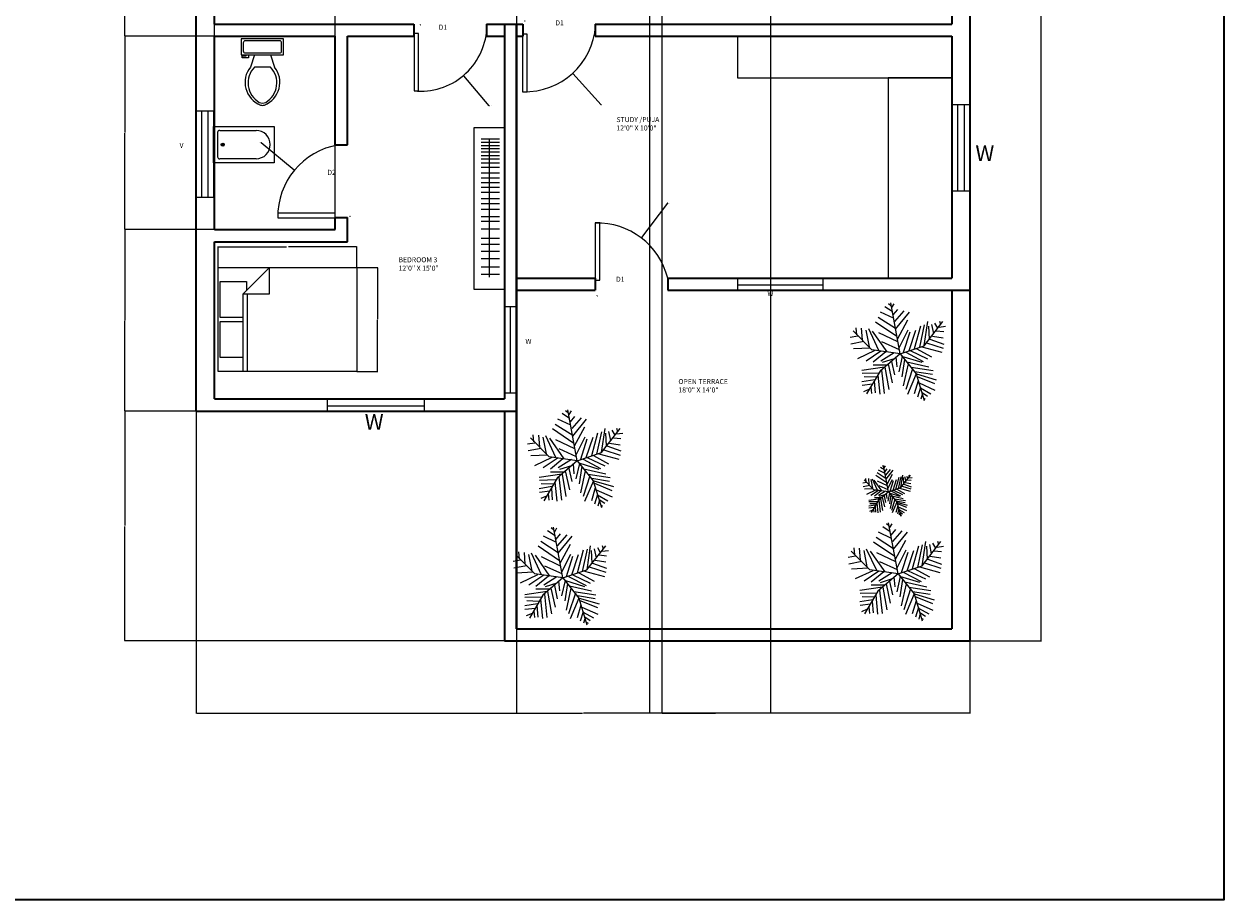
# Model space of a CAD drawing. Units: inches. Extents: x 65 to 1274, y 42 to 1041.
# Tile 4 of 6: x 678 to 1274, y 42 to 476. Entities that reach past the tile are written whole.
import ezdxf

# ---------------------------------------------------------------- set-up
doc = ezdxf.new("R2010")
doc.units = ezdxf.units.IN
for name, color, linetype, lineweight in [('A-ANNO-DIMS', 2, 'Continuous', 18), ('A-AREA-IDEN', 7, 'Continuous', 18), ('A-DOOR', 3, 'Continuous', 18), ('A-FLOR-CASE', 8, 'Continuous', 18), ('A-FLOR-FIXT', 9, 'Continuous', 18), ('A-FURN', 8, 'Continuous', 18), ('A-GLAZ', 4, 'Continuous', 18), ('A-WALL', 7, 'Continuous', 35), ('L-PLNT', 94, 'Continuous', 13), ('Text', 7, 'Continuous', 18), ('Title Block', 7, 'Continuous', 35)]:
    doc.layers.add(name, color=color, linetype=linetype, lineweight=lineweight)
doc.styles.get("Standard").update_dxf_attribs({"font": 'arial.ttf'})
doc.dimstyles.get("Standard").update_dxf_attribs({"dimtxt": 0.18, "dimasz": 0.18, "dimexe": 0.18, "dimexo": 0.0625, "dimgap": 0.09, "dimtad": 0, "dimtih": 1, "dimtoh": 1, "dimdec": 4, "dimzin": 0, "dimdsep": 46, "dimtxsty": 'Standard', "dimcen": 0.09, "dimadec": 0, "dimazin": 0, "dimtfac": 1, "dimtdec": 4, "dimtofl": 0, "dimtmove": 0, "dimatfit": 3, "dimfxl": 1, "dimtolj": 1, "dimtzin": 0, "dimarcsym": 0})

# ---------------------------------------------------------------- blocks, each defined once
blk = doc.blocks.new('Toilet - top')
for p, q in [((9.5, -6), (9.5, -2)), ((-10, -8.5), (-8, -8.5)), ((-10, -9.5), (-10, -8.5)), ((-7, -9.5), (-10, -9.5)), ((-8, -8.5), (-8, -8)), ((-7, -8), (-7, -9.5)), ((-4, -8), (-6, -14)), ((4, -8), (6, -14)), ((4, -14), (-4, -14))]:
    blk.add_line(p, q)
blk.add_lwpolyline([(10.5, -8), (10.5, 0), (-10.5, 0), (-10.5, -8)], close=True)
for points in [[(-9.5, -2), (-9.5, -6)], [(8.5, -1), (-8.5, -1)], [(-8.5, -7), (8.5, -7)]]:
    blk.add_lwpolyline(points)
for centre, radius, start, end in [((-8.62, -1.88), 0.884, 81.8699, 188.1301), ((8.62, -1.88), 0.884, 351.8699, 98.1301), ((-8.62, -6.12), 0.884, 171.8699, 278.1301), ((8.62, -6.12), 0.884, 261.8699, 8.1301), ((3.52, -21.58), 12.17, 141.46911, 247.97143), ((4.2, -21.82), 11.33, 136.36773, 238.94682), ((-3.52, -21.58), 12.17, 292.02843, 38.53071), ((-4.2, -21.82), 11.33, 301.05301, 43.63209), ((0, -27.88), 4, 245.73182, 294.26817), ((0, -29), 4, 254.86053, 285.13947)]:
    blk.add_arc(centre, radius, start, end)
blk = doc.blocks.new('Bath Tub - 26 x 60 in.')
for p, q in [((8, -18), (10, -18)), ((9, -17), (9, -19))]:
    blk.add_line(p, q)
blk.add_lwpolyline([(0, -36), (0, 0), (60, 0), (60, -36)], close=True)
for points in [[(4, -30), (4, -6)], [(6, -4), (42, -4)], [(42, -32), (6, -32)]]:
    blk.add_lwpolyline(points)
for radius in [1.5, 1]:
    blk.add_circle((9, -18), radius)
for centre, radius, start, end in [((5.75, -5.75), 1.77, 81.8699, 188.1301), ((42, -18), 14, 270, 90), ((5.75, -30.25), 1.77, 171.8699, 278.1301)]:
    blk.add_arc(centre, radius, start, end)
blk = doc.blocks.new('Bed - Queen')
for p, q in [((0, -80.00003), (0, 0)), ((0, 0), (59.99999, 0)), ((59.99999, 0), (59.99999, -80.00003)), ((7.99999, -1.2), (28.79998, -1.2)), ((7.99999, -14.4), (7.99999, -1.2)), ((28.79998, -1.2), (28.79998, -14.4)), ((31.19999, -1.2), (51.99999, -1.2)), ((31.19999, -14.4), (31.19999, -1.2)), ((51.99999, -1.2), (51.99999, -16.4)), ((0, -14.4), (44.8, -14.4)), ((44.8, -16.8), (0, -16.8)), ((59.99999, -29.6), (44.8, -14.4)), ((44.8, -14.4), (44.8, -29.6)), ((51.99999, -16.4), (46.79936, -16.4)), ((44.8, -29.6), (59.99999, -29.6)), ((59.99999, -80.00003), (0, -80.00003))]:
    blk.add_line(p, q)
blk = doc.blocks.new('*U4')
for p, q in [((-10.186, 53.64), (-13.084, 55.962)), ((0, 0), (-10.5, 57)), ((-9.099, 51.782), (-6.563, 55.962)), ((-5.114, 28.097), (-24.676, 40.636)), ((-7.288, 39.707), (-21.778, 46.673)), ((-8.737, 47.138), (-17.069, 52.711)), ((-7.65, 43.423), (-2.578, 49.46)), ((-5.839, 35.992), (4.667, 48.067)), ((-5.114, 27.632), (10.463, 46.673)), ((-48.585, 21.131), (-49.309, 29.026)), ((-43.513, 28.561), (-42.427, 15.558)), ((-35.544, 28.097), (-24.314, 3.947)), ((-3.665, 19.273), (-27.574, 35.527)), ((-2.941, 16.486), (8.652, 37.85)), ((16.259, 5.805), (23.142, 31.348)), ((22.055, 7.198), (27.489, 32.277)), ((27, 9), (48, 36)), ((27.127, 9.056), (31.112, 35.992)), ((31.836, 30.883), (32.561, 16.486)), ((35.096, 32.741), (37.27, 22.524)), ((38.719, 34.134), (41.979, 28.561)), ((43.791, 29.954), (51.036, 30.883)), ((44.153, 36.456), (45.239, 32.741)), ((-47.498, 19.737), (-55.83, 18.344)), ((-40.615, 13.7), (-55.105, 10.913)), ((-31.5, 4.5), (-52.5, 25.5)), ((-38.442, 26.239), (-34.819, 7.663)), ((-14.533, 2.09), (-30.834, 25.31)), ((-24.314, 23.917), (-2.941, 13.7)), ((-20.691, 13.7), (-1.129, 4.876)), ((-1.129, 6.734), (9.014, 26.704)), ((3.942, 1.625), (11.187, 24.381)), ((10.101, 3.483), (17.708, 26.239)), ((33.285, 16.486), (48.862, 10.913)), ((36.183, 19.737), (48.137, 17.88)), ((40.53, 25.775), (48.862, 24.846)), ((-33.37, 6.269), (-52.207, 5.34)), ((-28.299, 3.483), (-47.86, -5.805)), ((-21.416, 3.018), (-38.079, -8.128)), ((0, 0), (-31.5, 4.5)), ((-15.982, 2.09), (-30.11, -9.521)), ((0, 0), (-22.5, -19.5)), ((-6.563, 1.161), (-21.416, -8.128)), ((0, 0), (27, 9)), ((0, 0), (18, -22.5)), ((6.478, 1.625), (26.04, -8.592)), ((11.187, 3.483), (30.749, -5.805)), ((18.07, 5.805), (35.096, -3.483)), ((24.229, 7.663), (46.688, 1.625)), ((29.662, 12.307), (48.137, 6.269)), ((-15.257, -12.772), (-30.11, -12.772)), ((-6.563, -5.805), (-19.967, -9.985)), ((-13.446, -11.378), (-8.737, -32.741)), ((-9.461, -8.592), (-6.201, -23.453)), ((-4.752, -3.483), (-3.665, -14.629)), ((2.493, -3.019), (-1.491, -20.202)), ((1.769, -2.555), (24.229, -9.521)), ((5.029, -6.27), (2.131, -25.775)), ((9.014, -11.378), (3.58, -35.992)), ((7.565, -9.056), (32.198, -14.629)), ((-17.431, -15.094), (-42.789, -18.809)), ((-24.314, -21.596), (-42.427, -22.06)), ((-26.849, -26.24), (-40.253, -25.775)), ((-22.5, -19.5), (-37.5, -45)), ((-25.038, -23.918), (-22.865, -45.281)), ((-20.691, -18.345), (-17.793, -44.352)), ((-17.069, -15.094), (-12.721, -40.172)), ((14.085, -16.951), (6.478, -40.172)), ((18.07, -22.524), (8.289, -45.745)), ((12.274, -15.094), (36.907, -18.809)), ((16.259, -19.738), (36.183, -22.989)), ((18, -22.5), (27, -52.5)), ((18.433, -22.524), (40.53, -29.026)), ((19.157, -25.311), (38.719, -33.206)), ((-28.299, -29.026), (-42.789, -31.348)), ((-30.834, -34.135), (-42.427, -35.528)), ((-34.457, -39.708), (-40.978, -42.494)), ((-32.646, -36.921), (-31.921, -44.352)), ((-29.023, -30.884), (-27.936, -43.887)), ((20.244, -30.419), (15.897, -44.816)), ((22.78, -37.85), (19.519, -48.532)), ((21.331, -32.741), (39.081, -40.636)), ((22.78, -38.314), (34.372, -44.816)), ((24.591, -45.745), (23.142, -50.854)), ((24.591, -43.423), (30.749, -47.603)), ((26.764, -49.925), (28.213, -50.854))]:
    blk.add_line(p, q)
blk = doc.blocks.new('WIN-43-DEEP-FRAME')
for p, q in [((9, 42.65), (0, 42.65)), ((0, 42.65), (0, 0)), ((3, 0), (3, 42.65)), ((6, 42.65), (6, 0)), ((9, 0), (9, 42.65)), ((0, 0), (9, 0))]:
    blk.add_line(p, q)
blk = doc.blocks.new('*D30')
at = {"layer": 'A-ANNO-DIMS', "color": 0, "lineweight": -2, "transparency": 16777216}
for p, q in [((774.7, 355.42), (774.7, 365.85)), ((774.88, 365.67), (808.56, 365.67)), ((843.26, 365.67), (809.58, 365.67)), ((843.44, 355.42), (843.44, 365.85))]:
    blk.add_line(p, q, dxfattribs=at)
at = {"layer": 'A-ANNO-DIMS', "color": 0, "transparency": 16777216}
for points in [[(774.88, 365.7), (774.88, 365.64), (774.7, 365.67)], [(843.26, 365.7), (843.26, 365.64), (843.44, 365.67)]]:
    blk.add_solid(points, dxfattribs=at)
at = {"layer": 'Defpoints', "color": 0, "transparency": 16777216}
for p in [(774.7, 365.67), (774.7, 355.36), (843.44, 355.36)]:
    blk.add_point(p, dxfattribs=at)
at = {"layer": 'A-ANNO-DIMS', "color": 0, "transparency": 16777216, "insert": (809.07, 365.67), "char_height": 0.18, "attachment_point": 5}
blk.add_mtext('\\A1;BED 69', dxfattribs=at)
blk = doc.blocks.new('*D31')
at = {"layer": 'A-ANNO-DIMS', "color": 0, "lineweight": -2, "transparency": 16777216}
for p, q in [((843.5, 355.36), (853.93, 355.36)), ((853.75, 355.18), (853.75, 329.76)), ((853.75, 303.99), (853.75, 329.4)), ((843.5, 303.81), (853.93, 303.81))]:
    blk.add_line(p, q, dxfattribs=at)
at = {"layer": 'A-ANNO-DIMS', "color": 0, "transparency": 16777216}
for points in [[(853.72, 355.18), (853.78, 355.18), (853.75, 355.36)], [(853.72, 303.99), (853.78, 303.99), (853.75, 303.81)]]:
    blk.add_solid(points, dxfattribs=at)
at = {"layer": 'Defpoints', "color": 0, "transparency": 16777216}
for p in [(843.44, 355.36), (853.75, 355.36), (843.44, 303.81)]:
    blk.add_point(p, dxfattribs=at)
at = {"layer": 'A-ANNO-DIMS', "color": 0, "transparency": 16777216, "insert": (853.75, 329.58), "char_height": 0.18, "attachment_point": 5}
blk.add_mtext('\\A1;52', dxfattribs=at)
blk = doc.blocks.new('*D64')
at = {"layer": 'A-ANNO-DIMS', "color": 0, "lineweight": -2, "transparency": 16777216}
for p, q in [((763.83, 284.09), (763.83, 134.18)), ((1147.83, 170.09), (1147.83, 134.18)), ((764.01, 134.36), (955.54, 134.36)), ((1147.65, 134.36), (956.12, 134.36))]:
    blk.add_line(p, q, dxfattribs=at)
at = {"layer": 'A-ANNO-DIMS', "color": 0, "transparency": 16777216}
for points in [[(764.01, 134.39), (764.01, 134.33), (763.83, 134.36)], [(1147.65, 134.39), (1147.65, 134.33), (1147.83, 134.36)]]:
    blk.add_solid(points, dxfattribs=at)
at = {"layer": 'Defpoints', "color": 0, "transparency": 16777216}
for p in [(763.83, 284.15), (1147.83, 170.15), (1147.83, 134.36)]:
    blk.add_point(p, dxfattribs=at)
at = {"layer": 'A-ANNO-DIMS', "color": 0, "transparency": 16777216, "insert": (955.83, 134.36), "char_height": 0.18, "attachment_point": 5}
blk.add_mtext('\\A1;384', dxfattribs=at)
blk = doc.blocks.new('*D65')
at = {"layer": 'A-ANNO-DIMS', "color": 0, "lineweight": -2, "transparency": 16777216}
for p, q in [((1147.89, 827.15), (1183.32, 827.15)), ((1183.14, 826.97), (1183.14, 498.83)), ((1183.14, 170.33), (1183.14, 498.47)), ((1147.89, 170.15), (1183.32, 170.15))]:
    blk.add_line(p, q, dxfattribs=at)
at = {"layer": 'A-ANNO-DIMS', "color": 0, "transparency": 16777216}
for points in [[(1183.11, 826.97), (1183.17, 826.97), (1183.14, 827.15)], [(1183.11, 170.33), (1183.17, 170.33), (1183.14, 170.15)]]:
    blk.add_solid(points, dxfattribs=at)
at = {"layer": 'Defpoints', "color": 0, "transparency": 16777216}
for p in [(1147.83, 827.15), (1183.14, 827.15), (1147.83, 170.15)]:
    blk.add_point(p, dxfattribs=at)
at = {"layer": 'A-ANNO-DIMS', "color": 0, "transparency": 16777216, "insert": (1183.14, 498.65), "char_height": 0.18, "attachment_point": 5}
blk.add_mtext('\\A1;657', dxfattribs=at)
blk = doc.blocks.new('*D68')
at = {"layer": 'A-ANNO-DIMS', "color": 0, "lineweight": -2, "transparency": 16777216}
for p, q in [((922.83, 722.09), (922.83, 134.18)), ((988.83, 722.09), (988.83, 134.18)), ((923.01, 134.36), (955.61, 134.36)), ((988.65, 134.36), (956.05, 134.36))]:
    blk.add_line(p, q, dxfattribs=at)
at = {"layer": 'A-ANNO-DIMS', "color": 0, "transparency": 16777216}
for points in [[(923.01, 134.39), (923.01, 134.33), (922.83, 134.36)], [(988.65, 134.39), (988.65, 134.33), (988.83, 134.36)]]:
    blk.add_solid(points, dxfattribs=at)
at = {"layer": 'Defpoints', "color": 0, "transparency": 16777216}
for p in [(922.83, 722.15), (988.83, 722.15), (988.83, 134.36)]:
    blk.add_point(p, dxfattribs=at)
at = {"layer": 'A-ANNO-DIMS', "color": 0, "transparency": 16777216, "insert": (955.83, 134.36), "char_height": 0.18, "attachment_point": 5}
blk.add_mtext('\\A1;66', dxfattribs=at)
blk = doc.blocks.new('*D69')
at = {"layer": 'A-ANNO-DIMS', "color": 0, "lineweight": -2, "transparency": 16777216}
for p, q in [((994.83, 722.09), (994.83, 134.18)), ((1048.83, 722.09), (1048.83, 134.18)), ((995.01, 134.36), (1021.61, 134.36)), ((1048.65, 134.36), (1022.05, 134.36))]:
    blk.add_line(p, q, dxfattribs=at)
at = {"layer": 'A-ANNO-DIMS', "color": 0, "transparency": 16777216}
for points in [[(995.01, 134.39), (995.01, 134.33), (994.83, 134.36)], [(1048.65, 134.39), (1048.65, 134.33), (1048.83, 134.36)]]:
    blk.add_solid(points, dxfattribs=at)
at = {"layer": 'Defpoints', "color": 0, "transparency": 16777216}
for p in [(994.83, 722.15), (1048.83, 722.15), (1048.83, 134.36)]:
    blk.add_point(p, dxfattribs=at)
at = {"layer": 'A-ANNO-DIMS', "color": 0, "transparency": 16777216, "insert": (1021.83, 134.36), "char_height": 0.18, "attachment_point": 5}
blk.add_mtext('\\A1;54', dxfattribs=at)
blk = doc.blocks.new('*D70')
at = {"layer": 'A-ANNO-DIMS', "color": 0, "lineweight": -2, "transparency": 16777216}
for p, q in [((763.77, 284.15), (728.22, 284.15)), ((728.4, 283.97), (728.4, 227.33)), ((728.4, 170.33), (728.4, 226.97)), ((916.77, 170.15), (728.22, 170.15))]:
    blk.add_line(p, q, dxfattribs=at)
at = {"layer": 'A-ANNO-DIMS', "color": 0, "transparency": 16777216}
for points in [[(728.37, 283.97), (728.43, 283.97), (728.4, 284.15)], [(728.37, 170.33), (728.43, 170.33), (728.4, 170.15)]]:
    blk.add_solid(points, dxfattribs=at)
at = {"layer": 'Defpoints', "color": 0, "transparency": 16777216}
for p in [(728.4, 284.15), (763.83, 284.15), (916.83, 170.15)]:
    blk.add_point(p, dxfattribs=at)
at = {"layer": 'A-ANNO-DIMS', "color": 0, "transparency": 16777216, "insert": (728.4, 227.15), "char_height": 0.18, "attachment_point": 5}
blk.add_mtext('\\A1;114', dxfattribs=at)
blk = doc.blocks.new('*D71')
at = {"layer": 'A-ANNO-DIMS', "color": 0, "lineweight": -2, "transparency": 16777216}
for p, q in [((772.77, 374.15), (728.22, 374.15)), ((728.4, 373.97), (728.4, 329.33)), ((728.4, 284.33), (728.4, 328.97)), ((763.77, 284.15), (728.22, 284.15))]:
    blk.add_line(p, q, dxfattribs=at)
at = {"layer": 'A-ANNO-DIMS', "color": 0, "transparency": 16777216}
for points in [[(728.37, 373.97), (728.43, 373.97), (728.4, 374.15)], [(728.37, 284.33), (728.43, 284.33), (728.4, 284.15)]]:
    blk.add_solid(points, dxfattribs=at)
at = {"layer": 'Defpoints', "color": 0, "transparency": 16777216}
for p in [(728.4, 374.15), (772.83, 374.15), (763.83, 284.15)]:
    blk.add_point(p, dxfattribs=at)
at = {"layer": 'A-ANNO-DIMS', "color": 0, "transparency": 16777216, "insert": (728.4, 329.15), "char_height": 0.18, "attachment_point": 5}
blk.add_mtext('\\A1;90', dxfattribs=at)
blk = doc.blocks.new('*D72')
at = {"layer": 'A-ANNO-DIMS', "color": 0, "lineweight": -2, "transparency": 16777216}
for p, q in [((772.77, 470.15), (728.22, 470.15)), ((728.4, 469.97), (728.4, 422.33)), ((728.4, 374.33), (728.4, 421.97)), ((772.77, 374.15), (728.22, 374.15))]:
    blk.add_line(p, q, dxfattribs=at)
at = {"layer": 'A-ANNO-DIMS', "color": 0, "transparency": 16777216}
for points in [[(728.37, 469.97), (728.43, 469.97), (728.4, 470.15)], [(728.37, 374.33), (728.43, 374.33), (728.4, 374.15)]]:
    blk.add_solid(points, dxfattribs=at)
at = {"layer": 'Defpoints', "color": 0, "transparency": 16777216}
for p in [(728.4, 470.15), (772.83, 470.15), (772.83, 374.15)]:
    blk.add_point(p, dxfattribs=at)
at = {"layer": 'A-ANNO-DIMS', "color": 0, "transparency": 16777216, "insert": (728.4, 422.15), "char_height": 0.18, "attachment_point": 5}
blk.add_mtext('\\A1;96', dxfattribs=at)
blk = doc.blocks.new('*D73')
at = {"layer": 'A-ANNO-DIMS', "color": 0, "lineweight": -2, "transparency": 16777216}
for p, q in [((772.48, 549.58), (728.22, 549.58)), ((728.4, 549.4), (728.4, 510.05)), ((728.4, 470.33), (728.4, 509.68)), ((772.77, 470.15), (728.22, 470.15))]:
    blk.add_line(p, q, dxfattribs=at)
at = {"layer": 'A-ANNO-DIMS', "color": 0, "transparency": 16777216}
for points in [[(728.37, 549.4), (728.43, 549.4), (728.4, 549.58)], [(728.37, 470.33), (728.43, 470.33), (728.4, 470.15)]]:
    blk.add_solid(points, dxfattribs=at)
at = {"layer": 'Defpoints', "color": 0, "transparency": 16777216}
for p in [(728.4, 549.58), (772.55, 549.58), (772.83, 470.15)]:
    blk.add_point(p, dxfattribs=at)
at = {"layer": 'A-ANNO-DIMS', "color": 0, "transparency": 16777216, "insert": (728.4, 509.86), "char_height": 0.18, "attachment_point": 5}
blk.add_mtext('\\A1;79.43', dxfattribs=at)
blk = doc.blocks.new('*D77')
at = {"layer": 'A-ANNO-DIMS', "color": 0, "lineweight": -2, "transparency": 16777216}
for p, q in [((772.83, 374.21), (772.83, 890.96)), ((773.01, 890.78), (802.61, 890.78)), ((832.65, 890.78), (803.05, 890.78)), ((832.83, 374.21), (832.83, 890.96))]:
    blk.add_line(p, q, dxfattribs=at)
at = {"layer": 'A-ANNO-DIMS', "color": 0, "transparency": 16777216}
for points in [[(773.01, 890.81), (773.01, 890.75), (772.83, 890.78)], [(832.65, 890.81), (832.65, 890.75), (832.83, 890.78)]]:
    blk.add_solid(points, dxfattribs=at)
at = {"layer": 'Defpoints', "color": 0, "transparency": 16777216}
for p in [(832.83, 890.78), (772.83, 374.15), (832.83, 374.15)]:
    blk.add_point(p, dxfattribs=at)
at = {"layer": 'A-ANNO-DIMS', "color": 0, "transparency": 16777216, "insert": (802.83, 890.78), "char_height": 0.18, "attachment_point": 5}
blk.add_mtext('\\A1;60', dxfattribs=at)
blk = doc.blocks.new('*D84')
at = {"layer": 'A-ANNO-DIMS', "color": 0, "lineweight": -2, "transparency": 16777216}
for p, q in [((875.01, 475.78), (875.19, 475.78)), ((875.1, 475.69), (875.1, 475.87)), ((909.25, 435.54), (896.56, 450.49)), ((909.43, 435.54), (909.25, 435.54))]:
    blk.add_line(p, q, dxfattribs=at)
at = {"layer": 'A-ANNO-DIMS', "color": 0, "transparency": 16777216}
blk.add_solid([(896.59, 450.51), (896.54, 450.47), (896.45, 450.63)], dxfattribs=at)
at = {"layer": 'Defpoints', "color": 0, "transparency": 16777216}
for p in [(875.1, 475.78), (896.45, 450.63)]:
    blk.add_point(p, dxfattribs=at)
at = {"layer": 'A-ANNO-DIMS', "color": 0, "transparency": 16777216, "insert": (909.91, 435.54), "char_height": 0.18, "attachment_point": 5}
blk.add_mtext('\\A1;R32.99', dxfattribs=at)
blk = doc.blocks.new('*D85')
at = {"layer": 'A-ANNO-DIMS', "color": 0, "lineweight": -2, "transparency": 16777216}
for p, q in [((926.86, 477.66), (927.04, 477.66)), ((926.95, 477.57), (926.95, 477.75)), ((964.73, 436.07), (950.68, 451.53)), ((964.91, 436.07), (964.73, 436.07))]:
    blk.add_line(p, q, dxfattribs=at)
at = {"layer": 'A-ANNO-DIMS', "color": 0, "transparency": 16777216}
blk.add_solid([(950.7, 451.55), (950.66, 451.51), (950.56, 451.66)], dxfattribs=at)
at = {"layer": 'Defpoints', "color": 0, "transparency": 16777216}
for p in [(926.95, 477.66), (950.56, 451.66)]:
    blk.add_point(p, dxfattribs=at)
at = {"layer": 'A-ANNO-DIMS', "color": 0, "transparency": 16777216, "insert": (965.46, 436.07), "char_height": 0.18, "attachment_point": 5}
blk.add_mtext('\\A1;R35.115', dxfattribs=at)
blk = doc.blocks.new('*D86')
at = {"layer": 'A-ANNO-DIMS', "color": 0, "lineweight": -2, "transparency": 16777216}
for p, q in [((795.81, 417.41), (795.99, 417.41)), ((795.99, 417.41), (812.4, 403.79)), ((840.05, 380.78), (840.23, 380.78)), ((840.14, 380.69), (840.14, 380.87))]:
    blk.add_line(p, q, dxfattribs=at)
at = {"layer": 'A-ANNO-DIMS', "color": 0, "transparency": 16777216}
blk.add_solid([(812.42, 403.81), (812.39, 403.76), (812.54, 403.67)], dxfattribs=at)
at = {"layer": 'Defpoints', "color": 0, "transparency": 16777216}
for p in [(812.54, 403.67), (840.14, 380.78)]:
    blk.add_point(p, dxfattribs=at)
at = {"layer": 'A-ANNO-DIMS', "color": 0, "transparency": 16777216, "insert": (795.33, 417.41), "char_height": 0.18, "attachment_point": 5}
blk.add_mtext('\\A1;R35.86', dxfattribs=at)
blk = doc.blocks.new('*D87')
at = {"layer": 'A-ANNO-DIMS', "color": 0, "lineweight": -2, "transparency": 16777216}
for p, q in [((997.68, 387.33), (984.74, 370.24)), ((997.86, 387.33), (997.68, 387.33)), ((962.8, 341.38), (962.98, 341.38)), ((962.89, 341.29), (962.89, 341.47))]:
    blk.add_line(p, q, dxfattribs=at)
at = {"layer": 'A-ANNO-DIMS', "color": 0, "transparency": 16777216}
blk.add_solid([(984.72, 370.26), (984.77, 370.23), (984.63, 370.1)], dxfattribs=at)
at = {"layer": 'Defpoints', "color": 0, "transparency": 16777216}
for p in [(984.63, 370.1), (962.89, 341.38)]:
    blk.add_point(p, dxfattribs=at)
at = {"layer": 'A-ANNO-DIMS', "color": 0, "transparency": 16777216, "insert": (998.41, 387.33), "char_height": 0.18, "attachment_point": 5}
blk.add_mtext('\\A1;R36.025', dxfattribs=at)

msp = doc.modelspace()

# ---------------------------------------------------------------- linework, layer by layer
at = {"layer": 'A-DOOR'}
for points in [[(874.1798, 471.5069), (871.9224, 471.5069), (871.9224, 442.9853), (874.1798, 442.9853)], [(928.056, 471.0414), (925.7986, 471.0414), (925.7986, 442.5198), (928.056, 442.5198)], [(832.8244, 380.0252), (832.8244, 382.2826), (804.3028, 382.2826), (804.3028, 380.0252)], [(961.8654, 349.0583), (964.1227, 349.0583), (964.1227, 377.5799), (961.8654, 377.5799)]]:
    msp.add_lwpolyline(points, close=True, dxfattribs=at)
for centre, radius, start, end in [((875.1047, 475.7832), 32.989, 264.4081113, 356.2227601), ((926.948, 477.6553), 35.1155, 268.3281589, 356.1834795), ((840.1386, 380.7757), 35.857, 99.4299985, 181.2058247), ((962.8855, 341.3817), 36.0245, 14.007428, 91.7165176)]:
    msp.add_arc(centre, radius, start, end, dxfattribs=at)
at = {"layer": 'A-FLOR-CASE'}
for p, q in [((1032.4815, 469.8983), (1032.4815, 449.5036)), ((1032.4815, 449.5036), (1138.2983, 449.5036)), ((1138.2983, 449.5036), (1107.3091, 449.5036)), ((1107.3091, 449.5036), (1107.3091, 350.5513)), ((916.8328, 424.5951), (901.6677, 424.5951)), ((901.6677, 424.5951), (901.6677, 344.5544)), ((905.2602, 419.163), (914.3216, 419.163)), ((905.2602, 417.5927), (914.3216, 417.5927)), ((909.1466, 419.3923), (909.1466, 350.6252)), ((905.2602, 415.9643), (914.3216, 415.9643)), ((905.2602, 414.3941), (914.3216, 414.3941)), ((905.2602, 412.8239), (914.3216, 412.8239)), ((905.2602, 410.9047), (914.3216, 410.9047)), ((905.2602, 409.3345), (914.3216, 409.3345)), ((905.2602, 407.2408), (914.3216, 407.2408)), ((905.2602, 405.1472), (914.3216, 405.1472)), ((905.2602, 402.2975), (914.3216, 402.2975)), ((905.2602, 399.9131), (914.3216, 399.9131)), ((905.2602, 397.5868), (914.3216, 397.5868)), ((905.2602, 395.2605), (914.3216, 395.2605)), ((905.2602, 392.7016), (914.3216, 392.7016)), ((905.2602, 389.6711), (914.3216, 389.6711)), ((905.2602, 387.1598), (914.3216, 387.1598)), ((905.2602, 384.2765), (914.3216, 384.2765)), ((905.2602, 380.649), (914.3216, 380.649)), ((905.2602, 378.3238), (914.3216, 378.3238)), ((905.2602, 374.5103), (914.3216, 374.5103)), ((905.2602, 369.9528), (914.3216, 369.9528)), ((905.2602, 366.9764), (914.3216, 366.9764)), ((905.2602, 363.535), (914.3216, 363.535)), ((905.2602, 359.9076), (914.3216, 359.9076)), ((905.2602, 355.7221), (914.3216, 355.7221)), ((905.2602, 352.0947), (914.3216, 352.0947)), ((901.6677, 344.5544), (916.5959, 344.5544))]:
    msp.add_line(p, q, dxfattribs=at)
at = {"layer": 'A-GLAZ'}
for p, q in [((1032.3952, 349.7886), (1032.3952, 344.1476)), ((1075.0434, 349.7886), (1032.3952, 349.7886)), ((1032.3952, 346.7886), (1075.0434, 346.7886)), ((1075.0434, 344.1476), (1075.0434, 349.7886)), ((922.8297, 335.8095), (916.7273, 335.8095)), ((916.7273, 335.8095), (916.7273, 293.1613)), ((919.7273, 293.1613), (919.7273, 335.8095)), ((922.7273, 335.8095), (922.7273, 293.1613)), ((916.7273, 293.1613), (922.8297, 293.1613)), ((828.8468, 290.0688), (828.8468, 284.1476)), ((877.0151, 290.0688), (828.8468, 290.0688)), ((828.8468, 286.6805), (877.0151, 286.6805)), ((877.0151, 284.1476), (877.0151, 290.0688))]:
    msp.add_line(p, q, dxfattribs=at)
at = {"layer": 'A-WALL'}
for p, q in [((763.8297, 284.1476), (763.8297, 827.1476)), ((1147.8298, 827.1476), (1147.8298, 170.1476)), ((1138.8298, 716.1476), (1138.8298, 476.1476)), ((772.8297, 476.1476), (772.8297, 644.1476)), ((772.8297, 476.1476), (871.8298, 476.1476)), ((871.8298, 476.1476), (871.8298, 470.1476)), ((907.8298, 476.1476), (907.8298, 470.1476)), ((907.8298, 476.1476), (925.8298, 476.1476)), ((916.8297, 476.1476), (916.8297, 290.1476)), ((922.8297, 176.1476), (922.8297, 476.1476)), ((922.8297, 476.1476), (925.8298, 476.1476)), ((922.8297, 476.1476), (922.8297, 176.1476)), ((925.8298, 476.1476), (925.8298, 470.1476)), ((961.8298, 476.1476), (961.8298, 470.1476)), ((961.8298, 476.1476), (1138.8298, 476.1476)), ((772.8297, 470.1476), (832.8297, 470.1476)), ((772.8297, 374.1476), (772.8297, 470.1476)), ((832.8297, 416.1476), (832.8297, 470.1476)), ((838.8298, 416.1476), (838.8298, 470.1476)), ((838.8298, 470.1476), (871.8298, 470.1476)), ((907.8298, 470.1476), (916.8297, 470.1476)), ((922.8297, 470.1476), (925.8298, 470.1476)), ((922.8297, 470.1476), (925.8298, 470.1476)), ((961.8298, 470.1476), (1138.8298, 470.1476)), ((1138.8298, 470.1476), (1138.8298, 350.1476)), ((832.8297, 416.1476), (838.8298, 416.1476)), ((832.8297, 374.1476), (832.8297, 380.1476)), ((832.8297, 380.1476), (838.8298, 380.1476)), ((838.8298, 368.1476), (838.8298, 380.1476)), ((772.8297, 374.1476), (832.8297, 374.1476)), ((772.8297, 290.1476), (772.8297, 368.1476)), ((772.8297, 368.1476), (838.8298, 368.1476)), ((922.8297, 350.1476), (961.8298, 350.1476)), ((961.8298, 350.1476), (961.8298, 344.1476)), ((997.8298, 350.1476), (997.8298, 344.1476)), ((997.8298, 350.1476), (1138.8298, 350.1476)), ((922.8297, 344.1476), (961.8298, 344.1476)), ((997.8298, 344.1476), (1147.8298, 344.1476)), ((1138.8298, 344.1476), (1138.8298, 176.1476)), ((772.8297, 290.1476), (916.8297, 290.1476)), ((763.8297, 284.1476), (922.8297, 284.1476)), ((916.8297, 284.1476), (916.8297, 170.1476)), ((922.8297, 176.1476), (1138.8298, 176.1476)), ((916.8297, 170.1476), (1147.8298, 170.1476))]:
    msp.add_line(p, q, dxfattribs=at)
at = {"layer": 'Title Block'}
msp.add_lwpolyline([(64.7421, 1041.286), (1273.976, 1041.286), (1273.976, 41.6396), (64.7421, 41.6396)], close=True, dxfattribs=at)

# ---------------------------------------------------------------- block references
at = {"layer": 'A-FLOR-FIXT'}
msp.add_blockref('Toilet - top', (796.653, 468.7987), dxfattribs=at)
at = {"layer": 'A-FLOR-FIXT', "xscale": 0.5021616587859374, "yscale": 0.5021616587859374, "zscale": 0.5021616587859374}
msp.add_blockref('Bath Tub - 26 x 60 in.', (772.4159, 425.3723), dxfattribs=at)
at = {"layer": 'A-FURN', "xscale": 0.8592283626674893, "yscale": 0.8592283626674893, "zscale": 0.8592283626674893, "rotation": 89.99999999999999}
msp.add_blockref('Bed - Queen', (774.7035, 303.806), dxfattribs=at)
at = {"layer": 'A-GLAZ', "rotation": 180}
for p in [(1147.9215, 436.0488), (772.6012, 432.9737)]:
    msp.add_blockref('WIN-43-DEEP-FRAME', p, dxfattribs=at)
at = {"layer": 'L-PLNT'}
for p, xscale, yscale, zscale in [((1113.1818, 312.589), 0.4429176330503052, 0.4429176330503052, 0.4429176330503052), ((952.9234, 259.543), 0.4429176330503052, 0.4429176330503052, 0.4429176330503052), ((1107.412, 244.1247), 0.2291951906982327, 0.2291951906982327, 0.2291951906982327), ((945.7781, 201.3965), 0.4429176330503052, 0.4429176330503052, 0.4429176330503052), ((1112.161, 203.4367), 0.4429176330503052, 0.4429176330503052, 0.4429176330503052)]:
    msp.add_blockref('*U4', p, dxfattribs=dict(at, xscale=xscale, yscale=yscale, zscale=zscale))

# ---------------------------------------------------------------- texts
at = {"layer": 'A-AREA-IDEN', "char_height": 2.5, "attachment_point": 1}
for s, width, insert in [('STUDY /PUJA\\P12\'0" X 10\'0"', 60.794632, (972.3622, 430.0006)), ('BEDROOM 3\\P12\'0" X 15\'0"', 28.527606, (864.2114, 360.4523)), ('OPEN TERRACE\\P18\'0" X 14\'0"', 48.683115, (1003.1314, 300.0432))]:
    msp.add_mtext_dynamic_manual_height_columns(s, width=width, gutter_width=12.5, heights=[0], dxfattribs=dict(at, insert=insert))
at = {"layer": 'Text', "attachment_point": 1}
for s, width, gutter_width, insert, char_height in [('D1', 7.191641, 12.5, (942.0183, 477.9874), 2.5), ('D1', 11.448693, 12.5, (884.1232, 475.8214), 2.5), ('V', 5.099062, 12.5, (755.5155, 417.1893), 2.5), ('W', 96.254197, 39.1027, (1150.5703, 415.9814), 7.8205), ('D2', 12.419547, 12.5, (828.8683, 403.8236), 2.5), ('D1', 13.718662, 12.5, (972.1398, 350.7914), 2.5), ('W', 8.454515, 12.5, (1047.2936, 343.7643), 2.5), ('W', 14.031649, 12.5, (927.1989, 319.9479), 2.5), ('W', 96.254197, 39.1027, (847.4248, 282.6856), 7.8205)]:
    msp.add_mtext_dynamic_manual_height_columns(s, width=width, gutter_width=gutter_width, heights=[0], dxfattribs=dict(at, insert=insert, char_height=char_height))

# ---------------------------------------------------------------- dimensions: what is measured, and where the dimension line sits
at = {"layer": 'A-ANNO-DIMS'}
for base, p1, p2, picture, middle in [((832.8297, 890.7807), (772.8297, 374.1476), (832.8297, 374.1476), '*D77', (802.8297, 890.7807)), ((988.8297, 134.3565), (922.8297, 722.1476), (988.8297, 722.1476), '*D68', (955.8297, 134.3565)), ((1048.8298, 134.3565), (994.8297, 722.1476), (1048.8298, 722.1476), '*D69', (1021.8297, 134.3565)), ((1147.8298, 134.3565), (763.8297, 284.1476), (1147.8298, 170.1476), '*D64', (955.8297, 134.3565))]:
    dim = msp.add_linear_dim(base=base, p1=p1, p2=p2, dimstyle='Standard', override={"dimdec": 0, "dimlfac": 1, "dimrnd": 0, "dimzin": 0, "dimdsep": 46, "dimlunit": 2}, dxfattribs=at)
    dim.commit()
    dim.dimension.update_dxf_attribs({"geometry": picture, "text_midpoint": middle})
for base, p1, p2, override, picture, middle in [((1183.1357, 827.1476), (1147.8298, 170.1476), (1147.8298, 827.1476), {"dimdec": 0, "dimlfac": 1, "dimrnd": 0, "dimzin": 0, "dimdsep": 46, "dimlunit": 2}, '*D65', (1183.1357, 498.6476)), ((728.4012, 549.5812), (772.8297, 470.1476), (772.5457, 549.5812), {"dimdec": 2, "dimlfac": 1, "dimrnd": 0, "dimzin": 0, "dimdsep": 46, "dimlunit": 2}, '*D73', (728.4012, 509.8644)), ((728.4012, 470.1476), (772.8297, 374.1476), (772.8297, 470.1476), {"dimdec": 0, "dimlfac": 1, "dimrnd": 0, "dimzin": 0, "dimdsep": 46, "dimlunit": 2}, '*D72', (728.4012, 422.1476)), ((728.4012, 374.1476), (763.8297, 284.1476), (772.8297, 374.1476), {"dimdec": 0, "dimlfac": 1, "dimrnd": 0, "dimzin": 0, "dimdsep": 46, "dimlunit": 2}, '*D71', (728.4012, 329.1476)), ((853.7525, 355.3597), (843.4418, 303.806), (843.4418, 355.3597), {"dimdec": 0, "dimlfac": 1, "dimrnd": 0, "dimzin": 0, "dimdsep": 46, "dimlunit": 2}, '*D31', (853.7525, 329.5829)), ((728.4012, 284.1476), (916.8297, 170.1476), (763.8297, 284.1476), {"dimdec": 0, "dimlfac": 1, "dimrnd": 0, "dimzin": 0, "dimdsep": 46, "dimlunit": 2}, '*D70', (728.4012, 227.1476))]:
    dim = msp.add_linear_dim(base=base, p1=p1, p2=p2, angle=90, dimstyle='Standard', override=override, dxfattribs=at)
    dim.commit()
    dim.dimension.update_dxf_attribs({"geometry": picture, "text_midpoint": middle})
for center, mpoint, override, picture, middle in [((926.948, 477.6553), (950.5612, 451.6648), {"dimdec": 3, "dimlfac": 1, "dimrnd": 0, "dimzin": 0, "dimdsep": 46, "dimlunit": 2}, '*D85', (965.4596, 436.0704)), ((875.1047, 475.7832), (896.448, 450.629), {"dimdec": 2, "dimlfac": 1, "dimrnd": 0, "dimzin": 0, "dimdsep": 46, "dimlunit": 2}, '*D84', (909.9141, 435.5364)), ((840.1386, 380.7757), (812.5429, 403.6711), {"dimdec": 2, "dimlfac": 1, "dimrnd": 0, "dimzin": 0, "dimdsep": 46, "dimlunit": 2}, '*D86', (795.3257, 417.4083)), ((962.8855, 341.3817), (984.6349, 370.0998), {"dimdec": 3, "dimlfac": 1, "dimrnd": 0, "dimzin": 0, "dimdsep": 46, "dimlunit": 2}, '*D87', (998.4149, 387.3307))]:
    dim = msp.add_radius_dim(center=center, mpoint=mpoint, dimstyle='Standard', override=override, dxfattribs=at)
    dim.commit()
    dim.dimension.update_dxf_attribs({"geometry": picture, "text_midpoint": middle, "dimtype": 164})
dim = msp.add_linear_dim(base=(774.7035, 365.6705), p1=(843.4418, 355.3597), p2=(774.7035, 355.3597), angle=180, text='BED <>', dimstyle='Standard', override={"dimdec": 0, "dimlfac": 1, "dimrnd": 0, "dimzin": 0, "dimdsep": 46, "dimlunit": 2}, dxfattribs=at)
dim.commit()
dim.dimension.update_dxf_attribs({"geometry": '*D30', "text_midpoint": (809.0726, 365.6705)})

doc.saveas('drawing.dxf')
